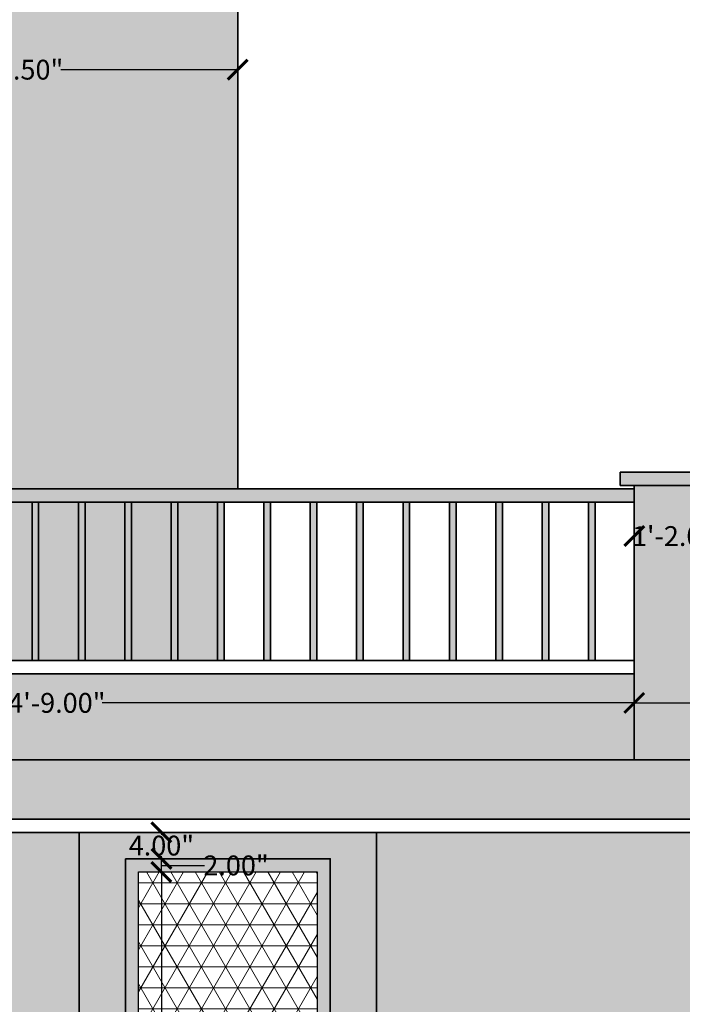
# Model space of a CAD drawing. Units: inches. Extents: x -654 to 390, y -40 to 648.
# Tile 11 of 13: x 92 to 192, y 417 to 566. Entities that reach past the tile are written whole.
import ezdxf

# ---------------------------------------------------------------- set-up
doc = ezdxf.new("R2010")
doc.units = ezdxf.units.IN
doc.header["$PDMODE"] = 3
for name, color, linetype, lineweight in [('A-ANNO-DIMS', 2, 'Continuous', 18), ('A-ELEV', 7, 'Continuous', 35), ('A-ELEV-FILL', 252, 'Continuous', 13), ('A-ELEV-PATT', 8, 'Continuous', 13), ('A-GLAZ', 4, 'Continuous', 25)]:
    doc.layers.add(name, color=color, linetype=linetype, lineweight=lineweight)
doc.styles.get("Standard").update_dxf_attribs({"font": 'arial.ttf'})
doc.dimstyles.get("Standard").update_dxf_attribs({"dimtxt": 3, "dimasz": 3, "dimexe": 0.18, "dimexo": 0.0625, "dimgap": 0.09, "dimtad": 0, "dimtih": 1, "dimtoh": 1, "dimzin": 0, "dimdsep": 46, "dimlunit": 3, "dimtxsty": 'Standard', "dimblk": 'ARCHTICK', "dimcen": 0.09, "dimse1": 1, "dimse2": 1, "dimadec": 0, "dimazin": 0, "dimtfac": 1, "dimtofl": 0, "dimtmove": 0, "dimatfit": 3, "dimfxl": 1, "dimtolj": 1, "dimtzin": 0, "dimarcsym": 0})

# ---------------------------------------------------------------- blocks, each defined once
blk = doc.blocks.new('_ArchTick')
at = {"color": 0, "linetype": 'ByBlock', "const_width": 0.15}
blk.add_lwpolyline([(-0.5, -0.5), (0.5, 0.5)], dxfattribs=at)
blk = doc.blocks.new('*D8')
at = {"layer": 'A-ANNO-DIMS', "color": 0, "lineweight": -2, "transparency": 16777216}
for p, q in [((360.51, 590.13), (360.51, 545.26)), ((360.51, 497.13), (360.51, 542.01))]:
    blk.add_line(p, q, dxfattribs=at)
at = {"layer": 'Defpoints', "color": 0, "transparency": 16777216}
for p in [(161.04, 590.13), (360.51, 590.13), (346.65, 497.13)]:
    blk.add_point(p, dxfattribs=at)
at = {"layer": 'A-ANNO-DIMS', "color": 0, "lineweight": -2, "transparency": 16777216, "xscale": 3, "yscale": 3, "zscale": 3}
for p, rotation in [((360.51, 590.13), 90), ((360.51, 497.13), 270)]:
    blk.add_blockref('_ArchTick', p, dxfattribs=dict(at, rotation=rotation))
at = {"layer": 'A-ANNO-DIMS', "color": 0, "transparency": 16777216, "insert": (360.51, 543.63), "char_height": 3, "attachment_point": 5}
blk.add_mtext('\\A1;7\'-9.00"', dxfattribs=at)
blk = doc.blocks.new('*D29')
at = {"layer": 'A-ANNO-DIMS', "color": 0, "lineweight": -2, "transparency": 16777216}
for p, q in [((57.15, 558.08), (83.91, 558.08)), ((124.65, 558.08), (97.89, 558.08))]:
    blk.add_line(p, q, dxfattribs=at)
at = {"layer": 'Defpoints', "color": 0, "transparency": 16777216}
for p in [(124.65, 558.08), (124.65, 558.08), (57.15, 546.63)]:
    blk.add_point(p, dxfattribs=at)
at = {"layer": 'A-ANNO-DIMS', "color": 0, "lineweight": -2, "transparency": 16777216, "xscale": 3, "yscale": 3, "zscale": 3, "rotation": 180}
blk.add_blockref('_ArchTick', (57.15, 558.08), dxfattribs=at)
at = {"layer": 'A-ANNO-DIMS', "color": 0, "lineweight": -2, "transparency": 16777216, "xscale": 3, "yscale": 3, "zscale": 3}
blk.add_blockref('_ArchTick', (124.65, 558.08), dxfattribs=at)
at = {"layer": 'A-ANNO-DIMS', "color": 0, "transparency": 16777216, "insert": (90.9, 558.08), "char_height": 3, "attachment_point": 5}
blk.add_mtext('\\A1;5\'-7.50"', dxfattribs=at)
blk = doc.blocks.new('*D31')
at = {"layer": 'A-ANNO-DIMS', "color": 0, "lineweight": -2, "transparency": 16777216}
for p, q in [((7.65, 462.23), (88.13, 462.23)), ((184.65, 462.23), (104.16, 462.23))]:
    blk.add_line(p, q, dxfattribs=at)
at = {"layer": 'Defpoints', "color": 0, "transparency": 16777216}
for p in [(7.65, 462.23), (184.65, 462.23), (184.65, 462.23)]:
    blk.add_point(p, dxfattribs=at)
at = {"layer": 'A-ANNO-DIMS', "color": 0, "lineweight": -2, "transparency": 16777216, "xscale": 3, "yscale": 3, "zscale": 3, "rotation": 180}
blk.add_blockref('_ArchTick', (7.65, 462.23), dxfattribs=at)
at = {"layer": 'A-ANNO-DIMS', "color": 0, "lineweight": -2, "transparency": 16777216, "xscale": 3, "yscale": 3, "zscale": 3}
blk.add_blockref('_ArchTick', (184.65, 462.23), dxfattribs=at)
at = {"layer": 'A-ANNO-DIMS', "color": 0, "transparency": 16777216, "insert": (96.15, 462.23), "char_height": 3, "attachment_point": 5}
blk.add_mtext('\\A1;14\'-9.00"', dxfattribs=at)
blk = doc.blocks.new('*D32')
at = {"layer": 'A-ANNO-DIMS', "color": 0, "lineweight": -2, "transparency": 16777216}
for p, q in [((184.65, 462.23), (257.63, 462.23)), ((346.65, 462.23), (273.66, 462.23))]:
    blk.add_line(p, q, dxfattribs=at)
at = {"layer": 'Defpoints', "color": 0, "transparency": 16777216}
for p in [(184.65, 462.23), (346.65, 462.23), (346.65, 462.23)]:
    blk.add_point(p, dxfattribs=at)
at = {"layer": 'A-ANNO-DIMS', "color": 0, "lineweight": -2, "transparency": 16777216, "xscale": 3, "yscale": 3, "zscale": 3, "rotation": 180}
blk.add_blockref('_ArchTick', (184.65, 462.23), dxfattribs=at)
at = {"layer": 'A-ANNO-DIMS', "color": 0, "lineweight": -2, "transparency": 16777216, "xscale": 3, "yscale": 3, "zscale": 3}
blk.add_blockref('_ArchTick', (346.65, 462.23), dxfattribs=at)
at = {"layer": 'A-ANNO-DIMS', "color": 0, "transparency": 16777216, "insert": (265.65, 462.23), "char_height": 3, "attachment_point": 5}
blk.add_mtext('\\A1;13\'-6.00"', dxfattribs=at)
blk = doc.blocks.new('*D37')
at = {"layer": 'A-ANNO-DIMS', "color": 0, "lineweight": -2, "transparency": 16777216}
for p, q in [((184.65, 487.48), (184.8, 487.48)), ((198.65, 487.48), (198.5, 487.48))]:
    blk.add_line(p, q, dxfattribs=at)
at = {"layer": 'Defpoints', "color": 0, "transparency": 16777216}
for p in [(184.65, 487.48), (184.65, 486.13), (198.65, 486.13)]:
    blk.add_point(p, dxfattribs=at)
at = {"layer": 'A-ANNO-DIMS', "color": 0, "lineweight": -2, "transparency": 16777216, "xscale": 3, "yscale": 3, "zscale": 3, "rotation": 180}
blk.add_blockref('_ArchTick', (184.65, 487.48), dxfattribs=at)
at = {"layer": 'A-ANNO-DIMS', "color": 0, "lineweight": -2, "transparency": 16777216, "xscale": 3, "yscale": 3, "zscale": 3}
blk.add_blockref('_ArchTick', (198.65, 487.48), dxfattribs=at)
at = {"layer": 'A-ANNO-DIMS', "color": 0, "transparency": 16777216, "insert": (191.65, 487.48), "char_height": 3, "attachment_point": 5}
blk.add_mtext('\\A1;1\'-2.00"', dxfattribs=at)
blk = doc.blocks.new('*D40')
at = {"layer": 'A-ANNO-DIMS', "color": 0, "lineweight": -2, "transparency": 16777216}
for p, q in [((230.97, 497.13), (230.97, 500.13)), ((230.97, 500.13), (233.97, 500.13)), ((230.97, 495.13), (230.97, 497.13))]:
    blk.add_line(p, q, dxfattribs=at)
at = {"layer": 'Defpoints', "color": 0, "transparency": 16777216}
for p in [(182.52, 497.13), (230.97, 497.13), (182.52, 495.13)]:
    blk.add_point(p, dxfattribs=at)
at = {"layer": 'A-ANNO-DIMS', "color": 0, "lineweight": -2, "transparency": 16777216, "xscale": 3, "yscale": 3, "zscale": 3}
for p, rotation in [((230.97, 497.13), 90), ((230.97, 495.13), 270)]:
    blk.add_blockref('_ArchTick', p, dxfattribs=dict(at, rotation=rotation))
at = {"layer": 'A-ANNO-DIMS', "color": 0, "transparency": 16777216, "insert": (238.72, 500.13), "char_height": 3, "attachment_point": 5}
blk.add_mtext('\\A1;2.00"', dxfattribs=at)
blk = doc.blocks.new('*D50')
at = {"layer": 'A-ANNO-DIMS', "color": 0, "lineweight": -2, "transparency": 16777216}
for p, q in [((113.1, 436.63), (113.1, 400.76)), ((113.1, 361.63), (113.1, 397.51))]:
    blk.add_line(p, q, dxfattribs=at)
at = {"layer": 'Defpoints', "color": 0, "transparency": 16777216}
for p in [(113.1, 436.63), (113.1, 436.63), (113.1, 361.63)]:
    blk.add_point(p, dxfattribs=at)
at = {"layer": 'A-ANNO-DIMS', "color": 0, "lineweight": -2, "transparency": 16777216, "xscale": 3, "yscale": 3, "zscale": 3}
for p, rotation in [((113.1, 436.63), 90), ((113.1, 361.63), 270)]:
    blk.add_blockref('_ArchTick', p, dxfattribs=dict(at, rotation=rotation))
at = {"layer": 'A-ANNO-DIMS', "color": 0, "transparency": 16777216, "insert": (113.1, 399.13), "char_height": 3, "attachment_point": 5}
blk.add_mtext('\\A1;6\'-3.00"', dxfattribs=at)
blk = doc.blocks.new('*D51')
at = {"layer": 'A-ANNO-DIMS', "color": 0, "lineweight": -2, "transparency": 16777216}
for p, q in [((113.1, 436.63), (113.1, 438.63)), ((113.1, 437.63), (119.45, 437.63)), ((119.45, 437.63), (119.63, 437.63))]:
    blk.add_line(p, q, dxfattribs=at)
at = {"layer": 'Defpoints', "color": 0, "transparency": 16777216}
for p in [(113.1, 438.63), (113.1, 438.63), (113.1, 436.63)]:
    blk.add_point(p, dxfattribs=at)
at = {"layer": 'A-ANNO-DIMS', "color": 0, "lineweight": -2, "transparency": 16777216, "xscale": 3, "yscale": 3, "zscale": 3}
for p, rotation in [((113.1, 438.63), 90), ((113.1, 436.63), 270)]:
    blk.add_blockref('_ArchTick', p, dxfattribs=dict(at, rotation=rotation))
at = {"layer": 'A-ANNO-DIMS', "color": 0, "transparency": 16777216, "insert": (124.39, 437.63), "char_height": 3, "attachment_point": 5}
blk.add_mtext('\\A1;2.00"', dxfattribs=at)
blk = doc.blocks.new('*D52')
at = {"layer": 'A-ANNO-DIMS', "color": 0, "lineweight": -2, "transparency": 16777216}
for p, q in [((113.1, 442.63), (113.1, 442.26)), ((113.1, 438.63), (113.1, 439.01))]:
    blk.add_line(p, q, dxfattribs=at)
at = {"layer": 'Defpoints', "color": 0, "transparency": 16777216}
for p in [(113.1, 442.63), (113.1, 442.63), (113.1, 438.63)]:
    blk.add_point(p, dxfattribs=at)
at = {"layer": 'A-ANNO-DIMS', "color": 0, "lineweight": -2, "transparency": 16777216, "xscale": 3, "yscale": 3, "zscale": 3}
for p, rotation in [((113.1, 442.63), 90), ((113.1, 438.63), 270)]:
    blk.add_blockref('_ArchTick', p, dxfattribs=dict(at, rotation=rotation))
at = {"layer": 'A-ANNO-DIMS', "color": 0, "transparency": 16777216, "insert": (113.1, 440.63), "char_height": 3, "attachment_point": 5}
blk.add_mtext('\\A1;4.00"', dxfattribs=at)
blk = doc.blocks.new('*D76')
at = {"layer": 'A-ANNO-DIMS', "color": 0, "lineweight": -2, "transparency": 16777216}
for p, q in [((380.75, 611.13), (380.75, 306.76)), ((380.75, -0.87), (380.75, 303.51))]:
    blk.add_line(p, q, dxfattribs=at)
at = {"layer": 'Defpoints', "color": 0, "transparency": 16777216}
for p in [(126.65, 611.13), (380.75, 611.13), (346.65, -0.87)]:
    blk.add_point(p, dxfattribs=at)
at = {"layer": 'A-ANNO-DIMS', "color": 0, "lineweight": -2, "transparency": 16777216, "xscale": 3, "yscale": 3, "zscale": 3}
for p, rotation in [((380.75, 611.13), 90), ((380.75, -0.87), 270)]:
    blk.add_blockref('_ArchTick', p, dxfattribs=dict(at, rotation=rotation))
at = {"layer": 'A-ANNO-DIMS', "color": 0, "transparency": 16777216, "insert": (380.75, 305.13), "char_height": 3, "attachment_point": 5}
blk.add_mtext('\\A1;51\'-0"', dxfattribs=at)
blk = doc.blocks.new('*D96')
at = {"layer": 'A-ANNO-DIMS', "color": 0, "lineweight": -2, "transparency": 16777216}
for p, q in [((128.74, 643.23), (130.74, 643.23)), ((130.74, 643.23), (133.74, 643.23))]:
    blk.add_line(p, q, dxfattribs=at)
at = {"layer": 'Defpoints', "color": 0, "transparency": 16777216}
for p in [(130.74, 643.23), (128.74, 311.13), (130.74, 311.13)]:
    blk.add_point(p, dxfattribs=at)
at = {"layer": 'A-ANNO-DIMS', "color": 0, "lineweight": -2, "transparency": 16777216, "xscale": 3, "yscale": 3, "zscale": 3, "rotation": 180}
blk.add_blockref('_ArchTick', (128.74, 643.23), dxfattribs=at)
at = {"layer": 'A-ANNO-DIMS', "color": 0, "lineweight": -2, "transparency": 16777216, "xscale": 3, "yscale": 3, "zscale": 3}
blk.add_blockref('_ArchTick', (130.74, 643.23), dxfattribs=at)
at = {"layer": 'A-ANNO-DIMS', "color": 0, "transparency": 16777216, "insert": (137.82, 643.23), "char_height": 3, "attachment_point": 5}
blk.add_mtext('\\A1;0\'-2"', dxfattribs=at)

msp = doc.modelspace()

# ---------------------------------------------------------------- hatches: boundary and pattern name
at = {"layer": 'A-ELEV-FILL'}
h = msp.add_hatch(color=256, dxfattribs=at)
h.dxf.hatch_style = 1
h.paths.add_polyline_path([(126.646, 611.134), (124.646, 611.134), (-1.354, 611.134), (-3.354, 611.134), (-3.354, 609.134), (-1.354, 609.134), (124.646, 609.134), (126.646, 609.134)])
h.paths.add_polyline_path([(8.646, 497.134), (-2.354, 497.134), (-2.354, 495.134), (8.646, 495.134)])
h.paths.add_polyline_path([(346.646, 497.134), (182.515, 497.134), (182.515, 495.134), (346.646, 495.134)])
h.paths.add_polyline_path([(198.646, 486.134), (198.646, 473.634), (209.366, 474.634), (199.646, 474.634), (199.646, 485.134), (209.366, 485.134)])
h.paths.add_polyline_path([(332.646, 486.134), (198.646, 486.134), (209.366, 485.134), (321.926, 485.134)])
h.paths.add_polyline_path([(321.926, 474.634), (209.366, 474.634), (198.646, 473.634), (332.646, 473.634)])
h.paths.add_polyline_path([(332.646, 486.134), (321.926, 485.134), (331.646, 485.134), (331.646, 474.634), (321.926, 474.634), (332.646, 473.634)])
h = msp.add_hatch(color=256, dxfattribs=at)
h.dxf.hatch_style = 1
h.paths.add_polyline_path([(115.646, 305.634), (97.646, 305.634), (97.646, 306.634), (98.293, 306.634), (98.293, 315.634), (97.646, 315.634), (97.646, 316.634), (100.646, 316.634), (100.646, 442.634), (-1.354, 442.634), (-1.354, 125.134), (115.646, 125.134)])
h.paths.add_polyline_path([(57.146, 161.134), (12.146, 161.134), (12.146, 413.134), (57.146, 413.134)], flags=16)
h.paths.add_polyline_path([(52.646, 165.634), (16.646, 165.634), (16.646, 408.634), (52.646, 408.634)], flags=0)
h.paths.add_polyline_path([(52.146, 166.134), (17.146, 166.134), (17.146, 408.134), (52.146, 408.134)], flags=0)
h.paths.add_polyline_path([(124.646, 581.134), (-1.354, 581.134), (-1.354, 497.134), (8.646, 497.134), (8.646, 494.634), (12.146, 494.634), (12.146, 546.634), (57.146, 546.634), (57.146, 494.634), (124.646, 494.634)])
h.paths.add_polyline_path([(124.646, 609.134), (-1.354, 609.134), (-1.354, 590.134), (124.646, 590.134)])
h = msp.add_hatch(color=256, dxfattribs=at)
h.dxf.hatch_style = 1
h.paths.add_polyline_path([(161.035, 590.134), (-1.354, 590.134), (-1.354, 581.134), (161.035, 581.134)])
h.paths.add_polyline_path([(346.646, 453.634), (-1.354, 453.634), (-1.354, 444.634), (337.646, 444.634), (337.646, 177.634), (178.742, 177.634), (178.742, 173.134), (176.742, 173.134), (176.742, 177.634), (166.742, 177.634), (166.742, 173.134), (164.742, 173.134), (164.742, 177.634), (154.742, 177.634), (154.742, 173.134), (152.742, 173.134), (152.742, 177.634), (142.742, 177.634), (142.742, 173.134), (140.742, 173.134), (140.742, 177.634), (130.742, 177.634), (130.742, 173.134), (128.742, 173.134), (128.742, 177.634), (115.646, 177.634), (115.646, 168.634), (346.646, 168.634), (346.646, 173.134)])
h.paths.add_polyline_path([(7.646, 87.642), (-1.354, 87.642), (-1.354, 17.134), (7.646, 17.134)])
h.paths.add_polyline_path([(16.396, 116.134), (60.646, 116.134), (60.646, 83.134), (62.646, 83.134), (113.646, 83.134), (115.646, 83.134), (115.646, 125.134), (7.646, 125.134), (7.646, 89.642), (8.146, 89.642), (8.146, 87.642), (7.646, 87.642), (7.646, 83.134), (9.646, 83.134), (16.396, 83.134)])
h = msp.add_hatch(color=256, dxfattribs=at)
h.dxf.hatch_style = 1
h.paths.add_polyline_path([(41.55, 80.08), (28.05, 80.08), (28.05, 20.08), (41.55, 20.08)])
h.paths.add_polyline_path([(93.843, 80.08), (80.343, 80.08), (80.343, 20.08), (93.843, 20.08)])
h.paths.add_polyline_path([(337.646, 442.634), (295.646, 442.634), (295.646, 316.634), (304.646, 316.634), (304.646, 315.634), (303.818, 315.634), (303.818, 306.634), (304.646, 306.634), (304.646, 305.634), (295.646, 305.634), (295.646, 177.634), (337.646, 177.634)])
h.paths.add_polyline_path([(346.646, 495.134), (184.646, 495.134), (184.646, 453.634), (346.646, 453.634)])
h.paths.add_polyline_path([(198.646, 473.634), (198.646, 486.134), (332.646, 486.134), (332.646, 473.634)], flags=16)
h.paths.add_polyline_path([(199.646, 474.634), (199.646, 485.134), (331.646, 485.134), (331.646, 474.634)], flags=0)
h = msp.add_hatch(color=256, dxfattribs=at)
h.dxf.hatch_style = 1
h.paths.add_polyline_path([(295.646, 190.634), (178.742, 190.634), (178.742, 177.634), (295.646, 177.634)])
h.paths.add_polyline_path([(176.742, 190.634), (166.742, 190.634), (166.742, 177.634), (176.742, 177.634)])
h.paths.add_polyline_path([(164.742, 190.634), (154.742, 190.634), (154.742, 177.634), (164.742, 177.634)])
h.paths.add_polyline_path([(152.742, 190.634), (142.742, 190.634), (142.742, 177.634), (152.742, 177.634)])
h.paths.add_polyline_path([(140.742, 190.634), (130.742, 190.634), (130.742, 177.634), (140.742, 177.634)])
h.paths.add_polyline_path([(128.742, 190.634), (120.146, 190.634), (120.146, 177.634), (128.742, 177.634)])
h.paths.add_polyline_path([(295.646, 329.634), (145.646, 329.634), (145.646, 442.634), (100.646, 442.634), (100.646, 316.634), (295.646, 316.634)])
h.paths.add_polyline_path([(138.646, 359.634), (107.646, 359.634), (107.646, 438.634), (138.646, 438.634)], flags=16)
h.paths.add_polyline_path([(136.646, 361.634), (109.646, 361.634), (109.646, 436.634), (136.646, 436.634)], flags=0)
h.paths.add_polyline_path([(184.646, 466.634), (7.646, 466.634), (7.646, 453.634), (184.646, 453.634)])
h.paths.add_polyline_path([(184.646, 494.634), (7.646, 494.634), (7.646, 492.634), (184.646, 492.634)])
h.paths.add_polyline_path([(10.336, 492.634), (9.336, 492.634), (9.336, 468.634), (10.336, 468.634)])
h.paths.add_polyline_path([(17.352, 492.634), (16.352, 492.634), (16.352, 468.634), (17.352, 468.634)])
h.paths.add_polyline_path([(24.368, 492.634), (23.368, 492.634), (23.368, 468.634), (24.368, 468.634)])
h.paths.add_polyline_path([(31.384, 492.634), (30.384, 492.634), (30.384, 468.634), (31.384, 468.634)])
h.paths.add_polyline_path([(38.4, 492.634), (37.4, 492.634), (37.4, 468.634), (38.4, 468.634)])
h.paths.add_polyline_path([(45.416, 492.634), (44.416, 492.634), (44.416, 468.634), (45.416, 468.634)])
h.paths.add_polyline_path([(52.432, 492.634), (51.432, 492.634), (51.432, 468.634), (52.432, 468.634)])
h.paths.add_polyline_path([(59.448, 492.634), (58.448, 492.634), (58.448, 468.634), (59.448, 468.634)])
h.paths.add_polyline_path([(66.464, 492.634), (65.464, 492.634), (65.464, 468.634), (66.464, 468.634)])
h.paths.add_polyline_path([(73.48, 492.634), (72.48, 492.634), (72.48, 468.634), (73.48, 468.634)])
h.paths.add_polyline_path([(80.496, 492.634), (79.496, 492.634), (79.496, 468.634), (80.496, 468.634)])
h.paths.add_polyline_path([(87.512, 492.634), (86.512, 492.634), (86.512, 468.634), (87.512, 468.634)])
h.paths.add_polyline_path([(94.528, 492.634), (93.528, 492.634), (93.528, 468.634), (94.528, 468.634)])
h.paths.add_polyline_path([(101.544, 492.634), (100.544, 492.634), (100.544, 468.634), (101.544, 468.634)])
h.paths.add_polyline_path([(108.559, 492.634), (107.559, 492.634), (107.559, 468.634), (108.559, 468.634)])
h.paths.add_polyline_path([(115.575, 492.634), (114.575, 492.634), (114.575, 468.634), (115.575, 468.634)])
h.paths.add_polyline_path([(122.591, 492.634), (121.591, 492.634), (121.591, 468.634), (122.591, 468.634)])
h.paths.add_polyline_path([(129.607, 492.634), (128.607, 492.634), (128.607, 468.634), (129.607, 468.634)])
h.paths.add_polyline_path([(136.623, 492.634), (135.623, 492.634), (135.623, 468.634), (136.623, 468.634)])
h.paths.add_polyline_path([(143.639, 492.634), (142.639, 492.634), (142.639, 468.634), (143.639, 468.634)])
h.paths.add_polyline_path([(150.655, 492.634), (149.655, 492.634), (149.655, 468.634), (150.655, 468.634)])
h.paths.add_polyline_path([(157.671, 492.634), (156.671, 492.634), (156.671, 468.634), (157.671, 468.634)])
h.paths.add_polyline_path([(164.687, 492.634), (163.687, 492.634), (163.687, 468.634), (164.687, 468.634)])
h.paths.add_polyline_path([(171.703, 492.634), (170.703, 492.634), (170.703, 468.634), (171.703, 468.634)])
h.paths.add_polyline_path([(178.719, 492.634), (177.719, 492.634), (177.719, 468.634), (178.719, 468.634)])
h = msp.add_hatch(color=256, dxfattribs=at)
h.dxf.hatch_style = 1
h.paths.add_polyline_path([(121.591, 492.634), (115.575, 492.634), (115.575, 468.634), (121.591, 468.634)])
h.paths.add_polyline_path([(114.575, 492.634), (108.559, 492.634), (108.559, 468.634), (114.575, 468.634)])
h.paths.add_polyline_path([(107.559, 492.634), (101.544, 492.634), (101.544, 468.634), (107.559, 468.634)])
h.paths.add_polyline_path([(100.544, 492.634), (94.528, 492.634), (94.528, 468.634), (100.544, 468.634)])
h.paths.add_polyline_path([(93.528, 492.634), (87.512, 492.634), (87.512, 468.634), (93.528, 468.634)])
h.paths.add_polyline_path([(86.512, 492.634), (80.496, 492.634), (80.496, 468.634), (86.512, 468.634)])
h.paths.add_polyline_path([(79.496, 492.634), (73.48, 492.634), (73.48, 468.634), (79.496, 468.634)])
h.paths.add_polyline_path([(72.48, 492.634), (66.464, 492.634), (66.464, 468.634), (72.48, 468.634)])
h.paths.add_polyline_path([(65.464, 492.634), (59.448, 492.634), (59.448, 468.634), (65.464, 468.634)])
h.paths.add_polyline_path([(58.448, 492.634), (57.146, 492.634), (57.146, 476.134), (52.432, 476.134), (52.432, 468.634), (58.448, 468.634)])
h.paths.add_polyline_path([(51.432, 476.134), (45.416, 476.134), (45.416, 468.634), (51.432, 468.634)])
h.paths.add_polyline_path([(44.416, 476.134), (38.4, 476.134), (38.4, 468.634), (44.416, 468.634)])
h.paths.add_polyline_path([(37.4, 476.134), (31.384, 476.134), (31.384, 468.634), (37.4, 468.634)])
h.paths.add_polyline_path([(30.384, 476.134), (24.368, 476.134), (24.368, 468.634), (30.384, 468.634)])
h.paths.add_polyline_path([(23.368, 476.134), (17.352, 476.134), (17.352, 468.634), (23.368, 468.634)])
h.paths.add_polyline_path([(16.352, 476.134), (12.146, 476.134), (12.146, 492.634), (10.336, 492.634), (10.336, 468.634), (16.352, 468.634)])
h.paths.add_polyline_path([(9.336, 492.634), (7.646, 492.634), (7.646, 468.634), (9.336, 468.634)])
h = msp.add_hatch(color=256, dxfattribs=at)
h.dxf.hatch_style = 1
h.paths.add_polyline_path([(239.871, 410.786), (291.141, 410.786), (291.141, 355.634), (295.646, 355.634), (295.646, 442.634), (145.646, 442.634), (145.646, 410.786), (179.877, 410.786), (179.877, 355.634), (239.871, 355.634)])
h = msp.add_hatch(color=256, dxfattribs=at)
h.dxf.hatch_style = 1
h.paths.add_polyline_path([(138.646, 438.634), (107.646, 438.634), (107.646, 359.634), (138.646, 359.634)])
h.paths.add_polyline_path([(136.646, 436.634), (136.646, 361.634), (109.646, 361.634), (109.646, 436.634)], flags=16)
h.paths.add_polyline_path([(179.877, 410.786), (145.646, 410.786), (145.646, 407.786), (153.285, 407.786), (153.285, 357.634), (145.646, 357.634), (145.646, 355.634), (179.877, 355.634)])
h.paths.add_polyline_path([(178.123, 407.786), (178.123, 357.634), (155.286, 357.634), (155.286, 407.786)], flags=16)
h.paths.add_polyline_path([(291.141, 410.786), (239.871, 410.786), (239.871, 355.634), (241.996, 355.634), (241.996, 407.786), (269.317, 407.786), (269.317, 355.634), (271.318, 355.634), (271.318, 407.786), (289.369, 407.786), (289.369, 355.634), (291.141, 355.634)])
h.paths.add_polyline_path([(128.225, 268.786), (128.742, 268.786), (128.742, 271.786), (125.225, 271.786), (125.225, 216.634), (128.225, 216.634)])
h.paths.add_polyline_path([(140.742, 271.786), (130.742, 271.786), (130.742, 268.786), (140.742, 268.786)])
h.paths.add_polyline_path([(152.742, 271.786), (142.742, 271.786), (142.742, 268.786), (152.742, 268.786)])
h.paths.add_polyline_path([(164.742, 271.786), (154.742, 271.786), (154.742, 268.786), (164.742, 268.786)])
h.paths.add_polyline_path([(176.742, 271.786), (167.328, 271.786), (166.742, 271.786), (166.742, 268.786), (167.328, 268.786), (167.328, 216.634), (169.328, 216.634), (169.328, 268.786), (176.742, 268.786)])
h.paths.add_polyline_path([(221.328, 271.786), (178.742, 271.786), (178.742, 268.786), (184.828, 268.786), (184.828, 216.634), (186.829, 216.634), (186.829, 268.786), (202.329, 268.786), (202.329, 216.634), (204.325, 216.634), (204.325, 268.786), (219.825, 268.786), (219.825, 216.634), (221.328, 216.634)])
h.paths.add_polyline_path([(295.646, 271.786), (244.726, 271.786), (244.726, 216.634), (246.481, 216.634), (246.481, 268.786), (269.317, 268.786), (269.317, 216.634), (271.318, 216.634), (271.318, 268.786), (286.818, 268.786), (286.818, 216.634), (288.814, 216.634), (288.814, 268.786), (295.646, 268.786)])
h.paths.add_polyline_path([(295.646, 216.634), (178.742, 216.634), (178.742, 214.634), (295.646, 214.634)])
h.paths.add_polyline_path([(128.742, 216.634), (123.485, 216.634), (123.485, 214.634), (128.742, 214.634)])
h.paths.add_polyline_path([(140.742, 216.634), (130.742, 216.634), (130.742, 214.634), (140.742, 214.634)])
h.paths.add_polyline_path([(152.742, 216.634), (142.742, 216.634), (142.742, 214.634), (152.742, 214.634)])
h.paths.add_polyline_path([(164.742, 216.634), (154.742, 216.634), (154.742, 214.634), (164.742, 214.634)])
h.paths.add_polyline_path([(176.742, 216.634), (166.742, 216.634), (166.742, 214.634), (176.742, 214.634)])
h.paths.add_polyline_path([(128.742, 192.634), (119.386, 192.634), (119.386, 190.634), (128.742, 190.634)])
h.paths.add_polyline_path([(140.742, 192.634), (130.742, 192.634), (130.742, 190.634), (140.742, 190.634)])
h.paths.add_polyline_path([(152.742, 192.634), (142.742, 192.634), (142.742, 190.634), (152.742, 190.634)])
h.paths.add_polyline_path([(164.742, 192.634), (154.742, 192.634), (154.742, 190.634), (164.742, 190.634)])
h.paths.add_polyline_path([(176.742, 192.634), (166.742, 192.634), (166.742, 190.634), (176.742, 190.634)])
h.paths.add_polyline_path([(295.646, 192.634), (178.742, 192.634), (178.742, 190.634), (295.646, 190.634)])
h.paths.add_polyline_path([(189.362, 137.63), (135.362, 137.63), (135.362, 71.63), (189.362, 71.63)])
h.paths.add_polyline_path([(154.862, 134.63), (170.362, 134.63), (170.362, 74.63), (154.862, 74.63)], flags=16)
h.paths.add_polyline_path([(152.862, 134.63), (152.862, 74.63), (137.362, 74.63), (137.362, 134.63)], flags=16)
h.paths.add_polyline_path([(172.358, 134.63), (187.858, 134.63), (187.858, 74.63), (172.358, 74.63)], flags=16)
h.paths.add_polyline_path([(113.646, 83.134), (62.646, 83.134), (62.646, 17.134), (113.646, 17.134)])
h.paths.add_polyline_path([(96.484, 80.08), (109.984, 80.08), (109.984, 20.08), (96.484, 20.08)], flags=16)
h.paths.add_polyline_path([(93.843, 80.08), (93.843, 20.08), (80.343, 20.08), (80.343, 80.08)], flags=16)
h.paths.add_polyline_path([(78.051, 80.08), (78.051, 20.08), (64.551, 20.08), (64.551, 80.08)], flags=16)
h.paths.add_polyline_path([(60.646, 83.134), (9.646, 83.134), (9.646, 17.134), (60.646, 17.134)])
h.paths.add_polyline_path([(58.197, 80.08), (58.197, 20.08), (44.697, 20.08), (44.697, 80.08)], flags=16)
h.paths.add_polyline_path([(41.55, 80.08), (41.55, 20.08), (28.05, 20.08), (28.05, 80.08)], flags=16)
h.paths.add_polyline_path([(25.146, 80.08), (25.146, 20.08), (11.646, 20.08), (11.646, 80.08)], flags=16)
h.paths.add_polyline_path([(9.646, 83.134), (7.646, 83.134), (7.646, 73.776), (9.646, 73.776)])
h.paths.add_polyline_path([(9.646, 65.663), (7.646, 65.663), (7.646, 36.041), (9.646, 36.041)])
h.paths.add_polyline_path([(9.646, 27.928), (7.646, 27.928), (7.646, 17.134), (9.646, 17.134)])
h.paths.add_polyline_path([(115.646, 83.134), (113.646, 83.134), (113.646, 73.776), (115.646, 73.776)])
h.paths.add_polyline_path([(115.646, 65.663), (113.646, 65.663), (113.646, 35.502), (115.646, 35.502)])
h.paths.add_polyline_path([(115.646, 27.389), (113.646, 27.389), (113.646, 17.134), (115.646, 17.134)])
h.paths.add_polyline_path([(8.146, 89.642), (-1.854, 89.642), (-1.854, 87.642), (8.146, 87.642)])
h.paths.add_polyline_path([(245.646, 156.634), (243.646, 156.634), (243.646, 17.134), (245.646, 17.134)])
h.paths.add_polyline_path([(339.646, 156.634), (337.646, 156.634), (337.646, 17.134), (339.646, 17.134)])
at = {"layer": 'A-ELEV-PATT'}
h = msp.add_hatch(dxfattribs=at)
h.set_pattern_fill('NET3', color=256)
h.paths.add_polyline_path([(136.646, 436.634), (109.646, 436.634), (109.646, 361.634), (136.646, 361.634)])

# ---------------------------------------------------------------- linework, layer by layer
at = {"layer": 'A-ELEV'}
for p, q in [((124.646, 581.134), (124.646, 494.634)), ((182.515, 495.134), (182.515, 497.134)), ((182.515, 497.134), (348.646, 497.134)), ((182.515, 495.134), (348.646, 495.134)), ((184.646, 453.634), (184.646, 495.134)), ((7.646, 494.634), (184.646, 494.634)), ((7.646, 492.634), (184.646, 492.634)), ((93.528, 492.634), (93.528, 468.634)), ((94.528, 492.634), (94.528, 468.634)), ((100.544, 492.634), (100.544, 468.634)), ((101.544, 492.634), (101.544, 468.634)), ((107.559, 492.634), (107.559, 468.634)), ((108.559, 492.634), (108.559, 468.634)), ((114.575, 492.634), (114.575, 468.634)), ((115.575, 492.634), (115.575, 468.634)), ((121.591, 492.634), (121.591, 468.634)), ((122.591, 492.634), (122.591, 468.634)), ((128.607, 492.634), (128.607, 468.634)), ((129.607, 492.634), (129.607, 468.634)), ((135.623, 492.634), (135.623, 468.634)), ((136.623, 492.634), (136.623, 468.634)), ((142.639, 492.634), (142.639, 468.634)), ((143.639, 492.634), (143.639, 468.634)), ((149.655, 492.634), (149.655, 468.634)), ((150.655, 492.634), (150.655, 468.634)), ((156.671, 492.634), (156.671, 468.634)), ((157.671, 492.634), (157.671, 468.634)), ((163.687, 492.634), (163.687, 468.634)), ((164.687, 492.634), (164.687, 468.634)), ((170.703, 492.634), (170.703, 468.634)), ((171.703, 492.634), (171.703, 468.634)), ((177.719, 492.634), (177.719, 468.634)), ((178.719, 492.634), (178.719, 468.634)), ((7.646, 468.634), (184.646, 468.634)), ((7.646, 466.634), (184.646, 466.634)), ((-1.354, 453.634), (346.646, 453.634)), ((7.646, 453.634), (184.646, 453.634)), ((-1.354, 444.634), (337.646, 444.634)), ((-1.354, 442.634), (337.646, 442.634)), ((100.646, 316.634), (100.646, 442.634)), ((145.646, 329.634), (145.646, 442.634))]:
    msp.add_line(p, q, dxfattribs=at)
msp.add_lwpolyline([(107.646, 438.634), (138.646, 438.634), (138.646, 359.634), (107.646, 359.634)], close=True, dxfattribs=at)
at = {"layer": 'A-GLAZ'}
msp.add_lwpolyline([(109.646, 436.634), (136.646, 436.634), (136.646, 361.634), (109.646, 361.634)], close=True, dxfattribs=at)

# ---------------------------------------------------------------- dimensions: what is measured, and where the dimension line sits
at = {"layer": 'A-ANNO-DIMS'}
for base, p1, p2, override, picture, middle in [((130.742, 643.234), (128.742, 311.134), (130.742, 311.134), {"dimdec": 1, "dimlfac": 1, "dimrnd": 0, "dimzin": 1, "dimdsep": 46, "dimlunit": 4, "dimfrac": 2}, '*D96', (137.82, 643.234)), ((124.646, 558.077), (57.146, 546.634), (124.646, 558.077), {"dimclrd": 0, "dimclre": 0, "dimclrt": 0, "dimtmove": 1}, '*D29', (90.896, 558.077)), ((184.646, 487.476), (198.646, 486.134), (184.646, 486.134), {"dimclrd": 0, "dimclre": 0, "dimclrt": 0}, '*D37', (191.646, 487.476)), ((184.646, 462.232), (7.646, 462.232), (184.646, 462.232), {"dimclrd": 0, "dimclre": 0, "dimclrt": 0}, '*D31', (96.146, 462.232)), ((346.646, 462.232), (184.646, 462.232), (346.646, 462.232), {"dimclrd": 0, "dimclre": 0, "dimclrt": 0, "dimtmove": 1}, '*D32', (265.646, 462.232))]:
    dim = msp.add_linear_dim(base=base, p1=p1, p2=p2, dimstyle='Standard', override=override, dxfattribs=at)
    dim.commit()
    dim.dimension.update_dxf_attribs({"geometry": picture, "text_midpoint": middle})
for base, p1, p2, override, picture, middle in [((380.746, 611.134), (346.646, -0.866), (126.646, 611.134), {"dimdec": 1, "dimlfac": 1, "dimrnd": 0, "dimzin": 1, "dimdsep": 46, "dimlunit": 4, "dimfrac": 2}, '*D76', (380.746, 305.134)), ((360.508, 590.134), (346.646, 497.134), (161.035, 590.134), {"dimclrd": 0, "dimclre": 0, "dimclrt": 0, "dimtmove": 1}, '*D8', (360.508, 543.634)), ((230.972, 497.134), (182.515, 495.134), (182.515, 497.134), {"dimclrd": 0, "dimclre": 0, "dimclrt": 0}, '*D40', (238.724, 500.134)), ((113.102, 442.634), (113.102, 438.634), (113.102, 442.634), {"dimclrd": 0, "dimclre": 0, "dimclrt": 0, "dimtmove": 1}, '*D52', (113.102, 440.634)), ((113.102, 438.634), (113.102, 436.634), (113.102, 438.634), {"dimclrd": 0, "dimclre": 0, "dimclrt": 0, "dimtmove": 1}, '*D51', (119.724, 437.634)), ((113.102, 436.634), (113.102, 361.634), (113.102, 436.634), {"dimclrd": 0, "dimclre": 0, "dimclrt": 0, "dimtmove": 1}, '*D50', (113.102, 399.134))]:
    dim = msp.add_linear_dim(base=base, p1=p1, p2=p2, angle=90, dimstyle='Standard', override=override, dxfattribs=at)
    dim.commit()
    dim.dimension.update_dxf_attribs({"geometry": picture, "text_midpoint": middle})

doc.saveas('drawing.dxf')
